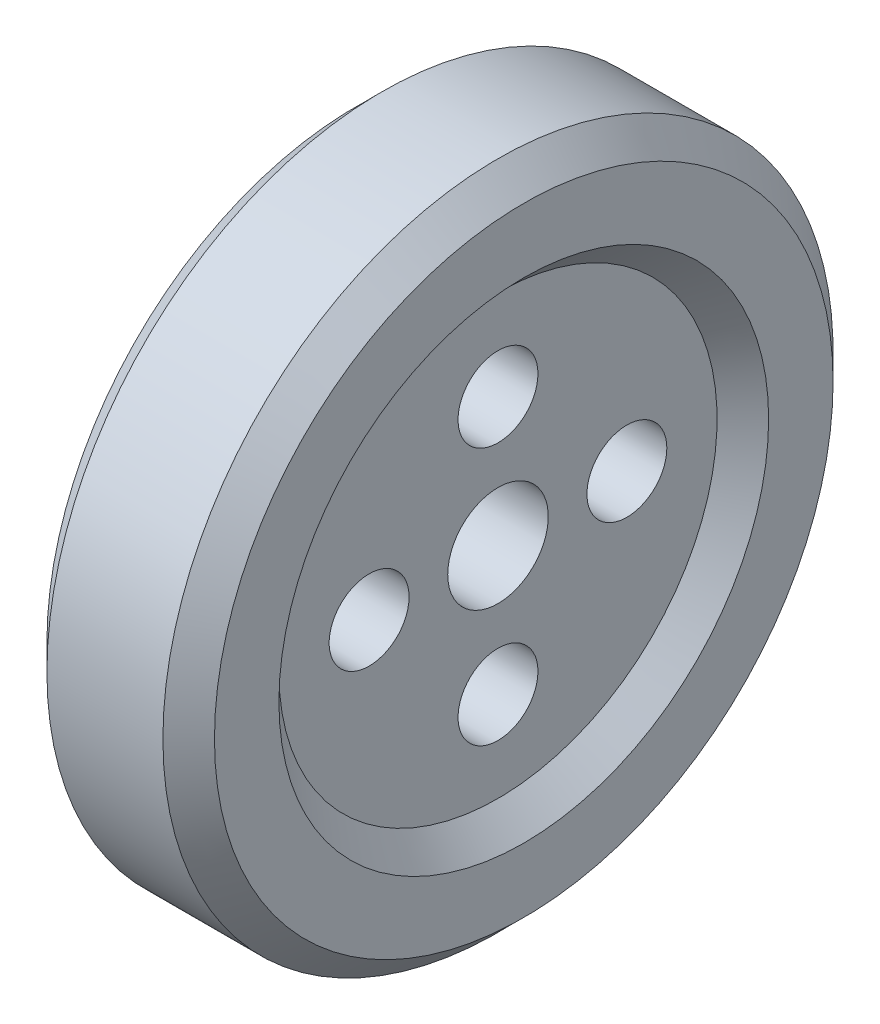
SolidWorks part; units mm, degrees
material "Plain Carbon Steel"
ref_plane "Front Plane" through (0, 0, 0) normal (0, 0, 1) x (1, 0, 0)
ref_plane "Top Plane" through (0, 0, 0) normal (0, 1, 0) x (1, 0, 0)
ref_plane "Right Plane" through (0, 0, 0) normal (1, 0, 0) x (0, 0, -1)
sketch "Disc Profile Sketch" plane through (0, 0, 0) normal (0, 0, 1) x (1, 0, 0)
  line L0 (-45, 260) -> (-65, 240)
  line L1 (45, 260) -> (-45, 260)
  line L2 (65, 240) -> (65, 190)
  line L4 (-65, 240) -> (-65, 190)
  line L5 (65, 240) -> (45, 260)
  line L6 (-186.1159, 0) -> (142.1578, 0) construction
  line L9 (45, 170) -> (45, 39)
  line L11 (-45, 170) -> (-45, 39)
  line L12 (45, 39) -> (-45, 39)
  line L15 (-65, 190) -> (-45, 170)
  line L16 (65, 190) -> (45, 170)
  point P0 (0, 0)
  point P2 (65, 260)
  point P4 (-65, 260)
  point P10 (0, 260)
  point P14 (0, 0)
  point P20 (0, 0)
  dimension "D1" = 130
  dimension "D2" = 260
  dimension "D3" = 50
  dimension "D4" = 131
revolve "Button Disc Body" add sketch "Disc Profile Sketch" angle 360 about L6
sketch "Thread Holes Sketch" plane through (45, 0, 0) normal (1, 0, 0) x (0, 0, -1)
  circle A0 centre (0, 100) radius 31
  circle A1 centre (100, 0) radius 31
  circle A2 centre (0, -100) radius 31
  circle A3 centre (-100, 0) radius 31
  circle A4 centre (0, 0) radius 170 construction
  point P12 (0, 0)
  dimension "D1" = 62
  dimension "D2" = 100
  dimension "D4" = 100
  dimension "D5" = 100
  dimension "D3" = 4
extrude "Thread Holes 5x" cut sketch "Thread Holes Sketch" against normal up to next
